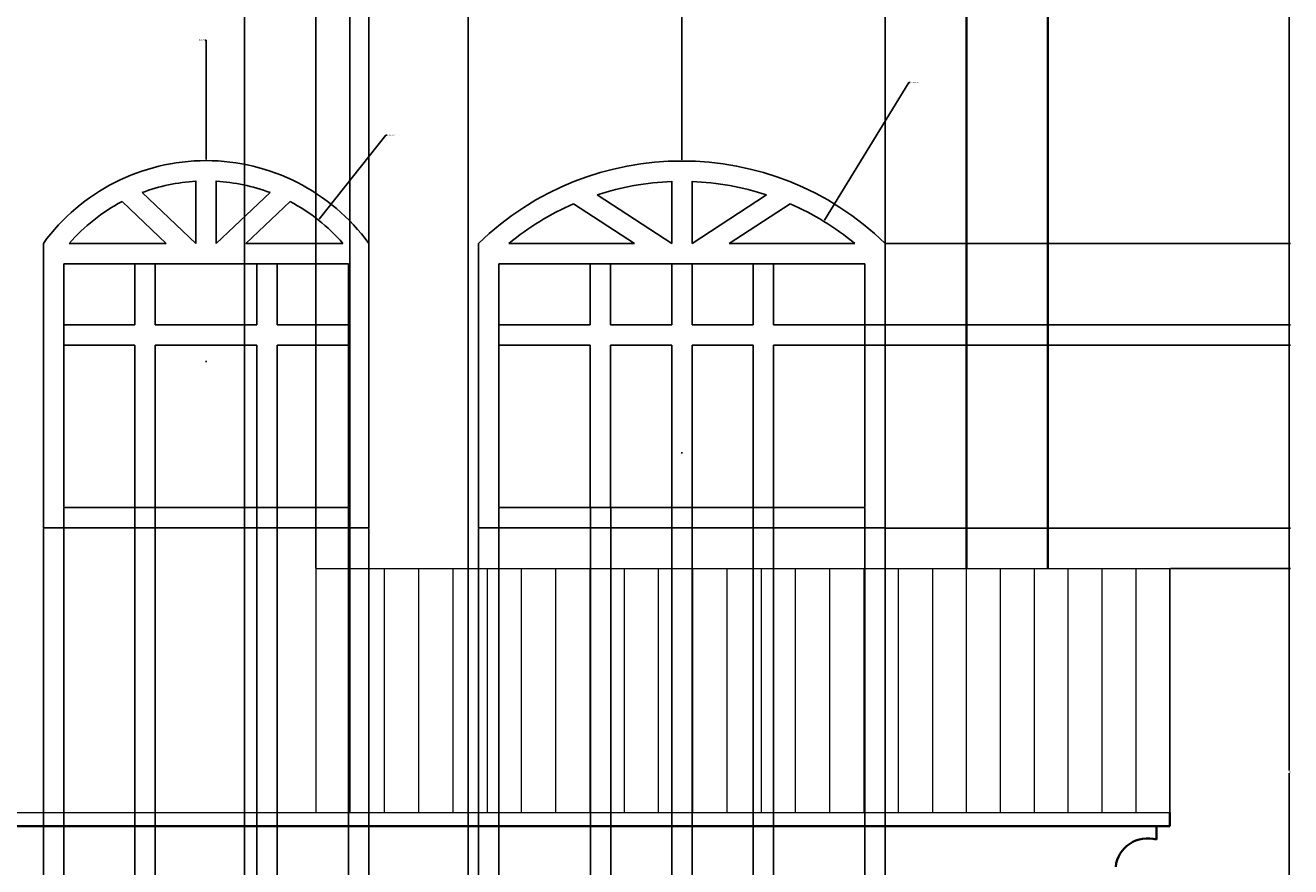
# Model space of a CAD drawing. Units: inches. Extents: x 2612 to 2948, y 481 to 865.
# Tile 6 of 7: x 2761 to 2948, y 659 to 783. Entities that reach past the tile are written whole.
import ezdxf

# ---------------------------------------------------------------- set-up
doc = ezdxf.new("R2010")
doc.units = ezdxf.units.IN
for name, color, linetype, lineweight in [('A-ANNO-DIMS', 2, 'Continuous', 18), ('A-COLS', 1, 'Continuous', 35), ('A-ELEV', 7, 'Continuous', 35), ('A-ELEV-RAIL', 3, 'Continuous', 18), ('A-GLAZ', 4, 'Continuous', 25)]:
    doc.layers.add(name, color=color, linetype=linetype, lineweight=lineweight)
doc.styles.get("Standard").update_dxf_attribs({"font": 'arial.ttf'})
doc.dimstyles.get("Standard").update_dxf_attribs({"dimtxt": 0.18, "dimasz": 0.18, "dimexe": 0.18, "dimexo": 0.0625, "dimgap": 0.09, "dimtad": 0, "dimtih": 1, "dimtoh": 1, "dimdec": 4, "dimzin": 0, "dimdsep": 46, "dimtxsty": 'Standard', "dimcen": 0.09, "dimadec": 0, "dimazin": 0, "dimtfac": 1, "dimtdec": 4, "dimtofl": 0, "dimtmove": 0, "dimatfit": 3, "dimfxl": 1, "dimtolj": 1, "dimtzin": 0, "dimarcsym": 0})

# ---------------------------------------------------------------- blocks, each defined once
blk = doc.blocks.new('*D15')
at = {"layer": 'A-ANNO-DIMS', "color": 0, "lineweight": -2, "transparency": 16777216}
for p, q in [((2888.37, 709.04), (2948.09, 709.04)), ((2947.91, 708.86), (2947.91, 706.23)), ((2947.91, 703.22), (2947.91, 705.86)), ((2930.37, 703.04), (2948.09, 703.04))]:
    blk.add_line(p, q, dxfattribs=at)
at = {"layer": 'A-ANNO-DIMS', "color": 0, "transparency": 16777216}
for points in [[(2947.88, 708.86), (2947.94, 708.86), (2947.91, 709.04)], [(2947.88, 703.22), (2947.94, 703.22), (2947.91, 703.04)]]:
    blk.add_solid(points, dxfattribs=at)
at = {"layer": 'Defpoints', "color": 0, "transparency": 16777216}
for p in [(2888.31, 709.04), (2947.91, 709.04), (2930.31, 703.04)]:
    blk.add_point(p, dxfattribs=at)
at = {"layer": 'A-ANNO-DIMS', "color": 0, "transparency": 16777216, "insert": (2947.91, 706.04), "char_height": 0.18, "attachment_point": 5}
blk.add_mtext('\\A1;6', dxfattribs=at)
blk = doc.blocks.new('*D33')
at = {"layer": 'A-ANNO-DIMS', "color": 0, "lineweight": -2, "transparency": 16777216}
for p, q in [((2756.31, 703.11), (2756.31, 864.82)), ((2756.49, 864.64), (2780.08, 864.64)), ((2804.13, 864.64), (2780.53, 864.64)), ((2804.31, 703.11), (2804.31, 864.82))]:
    blk.add_line(p, q, dxfattribs=at)
at = {"layer": 'A-ANNO-DIMS', "color": 0, "transparency": 16777216}
for points in [[(2756.49, 864.67), (2756.49, 864.61), (2756.31, 864.64)], [(2804.13, 864.67), (2804.13, 864.61), (2804.31, 864.64)]]:
    blk.add_solid(points, dxfattribs=at)
at = {"layer": 'Defpoints', "color": 0, "transparency": 16777216}
for p in [(2804.31, 864.64), (2756.31, 703.04), (2804.31, 703.04)]:
    blk.add_point(p, dxfattribs=at)
at = {"layer": 'A-ANNO-DIMS', "color": 0, "transparency": 16777216, "insert": (2780.31, 864.64), "char_height": 0.18, "attachment_point": 5}
blk.add_mtext('\\A1;48', dxfattribs=at)
blk = doc.blocks.new('*D34')
at = {"layer": 'A-ANNO-DIMS', "color": 0, "lineweight": -2, "transparency": 16777216}
for p, q in [((2804.31, 703.11), (2804.31, 864.82)), ((2804.49, 864.64), (2806.44, 864.64)), ((2809.18, 864.64), (2807.23, 864.64)), ((2809.36, 703.11), (2809.36, 864.82))]:
    blk.add_line(p, q, dxfattribs=at)
at = {"layer": 'A-ANNO-DIMS', "color": 0, "transparency": 16777216}
for points in [[(2804.49, 864.67), (2804.49, 864.61), (2804.31, 864.64)], [(2809.18, 864.67), (2809.18, 864.61), (2809.36, 864.64)]]:
    blk.add_solid(points, dxfattribs=at)
at = {"layer": 'Defpoints', "color": 0, "transparency": 16777216}
for p in [(2809.36, 864.64), (2804.31, 703.04), (2809.36, 703.04)]:
    blk.add_point(p, dxfattribs=at)
at = {"layer": 'A-ANNO-DIMS', "color": 0, "transparency": 16777216, "insert": (2806.83, 864.64), "char_height": 0.18, "attachment_point": 5}
blk.add_mtext('\\A1;5.053', dxfattribs=at)
blk = doc.blocks.new('*D35')
at = {"layer": 'A-ANNO-DIMS', "color": 0, "lineweight": -2, "transparency": 16777216}
for p, q in [((2809.36, 703.11), (2809.36, 864.82)), ((2809.54, 864.64), (2810.42, 864.64)), ((2811.95, 864.64), (2811.07, 864.64)), ((2812.13, 709.11), (2812.13, 864.82))]:
    blk.add_line(p, q, dxfattribs=at)
at = {"layer": 'A-ANNO-DIMS', "color": 0, "transparency": 16777216}
for points in [[(2809.54, 864.67), (2809.54, 864.61), (2809.36, 864.64)], [(2811.95, 864.67), (2811.95, 864.61), (2812.13, 864.64)]]:
    blk.add_solid(points, dxfattribs=at)
at = {"layer": 'Defpoints', "color": 0, "transparency": 16777216}
for p in [(2812.13, 864.64), (2812.13, 709.04), (2809.36, 703.04)]:
    blk.add_point(p, dxfattribs=at)
at = {"layer": 'A-ANNO-DIMS', "color": 0, "transparency": 16777216, "insert": (2810.75, 864.64), "char_height": 0.18, "attachment_point": 5}
blk.add_mtext('\\A1;2.77', dxfattribs=at)
blk = doc.blocks.new('*D36')
at = {"layer": 'A-ANNO-DIMS', "color": 0, "lineweight": -2, "transparency": 16777216}
for p, q in [((2888.31, 709.11), (2888.31, 864.82)), ((2888.49, 864.64), (2894.1, 864.64)), ((2900.13, 864.64), (2894.52, 864.64)), ((2900.31, 787.11), (2900.31, 864.82))]:
    blk.add_line(p, q, dxfattribs=at)
at = {"layer": 'A-ANNO-DIMS', "color": 0, "transparency": 16777216}
for points in [[(2888.49, 864.67), (2888.49, 864.61), (2888.31, 864.64)], [(2900.13, 864.67), (2900.13, 864.61), (2900.31, 864.64)]]:
    blk.add_solid(points, dxfattribs=at)
at = {"layer": 'Defpoints', "color": 0, "transparency": 16777216}
for p in [(2900.31, 864.64), (2900.31, 787.04), (2888.31, 709.04)]:
    blk.add_point(p, dxfattribs=at)
at = {"layer": 'A-ANNO-DIMS', "color": 0, "transparency": 16777216, "insert": (2894.31, 864.64), "char_height": 0.18, "attachment_point": 5}
blk.add_mtext('\\A1;12', dxfattribs=at)
blk = doc.blocks.new('*D50')
at = {"layer": 'A-ANNO-DIMS', "color": 0, "lineweight": -2, "transparency": 16777216}
for p, q in [((2745.81, 604.11), (2745.81, 864.82)), ((2745.99, 864.64), (2769.58, 864.64)), ((2793.63, 864.64), (2770.03, 864.64)), ((2793.81, 604.11), (2793.81, 864.82))]:
    blk.add_line(p, q, dxfattribs=at)
at = {"layer": 'A-ANNO-DIMS', "color": 0, "transparency": 16777216}
for points in [[(2745.99, 864.67), (2745.99, 864.61), (2745.81, 864.64)], [(2793.63, 864.67), (2793.63, 864.61), (2793.81, 864.64)]]:
    blk.add_solid(points, dxfattribs=at)
at = {"layer": 'Defpoints', "color": 0, "transparency": 16777216}
for p in [(2793.81, 864.64), (2745.81, 604.04), (2793.81, 604.04)]:
    blk.add_point(p, dxfattribs=at)
at = {"layer": 'A-ANNO-DIMS', "color": 0, "transparency": 16777216, "insert": (2769.81, 864.64), "char_height": 0.18, "attachment_point": 5}
blk.add_mtext('\\A1;48', dxfattribs=at)
blk = doc.blocks.new('*D51')
at = {"layer": 'A-ANNO-DIMS', "color": 0, "lineweight": -2, "transparency": 16777216}
for p, q in [((2793.81, 604.11), (2793.81, 864.82)), ((2793.99, 864.64), (2810.09, 864.64)), ((2826.63, 864.64), (2810.53, 864.64)), ((2826.81, 562.11), (2826.81, 864.82))]:
    blk.add_line(p, q, dxfattribs=at)
at = {"layer": 'A-ANNO-DIMS', "color": 0, "transparency": 16777216}
for points in [[(2793.99, 864.67), (2793.99, 864.61), (2793.81, 864.64)], [(2826.63, 864.67), (2826.63, 864.61), (2826.81, 864.64)]]:
    blk.add_solid(points, dxfattribs=at)
at = {"layer": 'Defpoints', "color": 0, "transparency": 16777216}
for p in [(2826.81, 864.64), (2793.81, 604.04), (2826.81, 562.04)]:
    blk.add_point(p, dxfattribs=at)
at = {"layer": 'A-ANNO-DIMS', "color": 0, "transparency": 16777216, "insert": (2810.31, 864.64), "char_height": 0.18, "attachment_point": 5}
blk.add_mtext('\\A1;33', dxfattribs=at)
blk = doc.blocks.new('*D66')
at = {"layer": 'A-ANNO-DIMS', "color": 0, "lineweight": -2, "transparency": 16777216}
for p, q in [((2767.13, 711.98), (2767.13, 481.26)), ((2764.13, 708.98), (2764.13, 481.26)), ((2764.31, 481.44), (2765.48, 481.44)), ((2766.95, 481.44), (2765.78, 481.44))]:
    blk.add_line(p, q, dxfattribs=at)
at = {"layer": 'A-ANNO-DIMS', "color": 0, "transparency": 16777216}
for points in [[(2764.31, 481.47), (2764.31, 481.41), (2764.13, 481.44)], [(2766.95, 481.47), (2766.95, 481.41), (2767.13, 481.44)]]:
    blk.add_solid(points, dxfattribs=at)
at = {"layer": 'Defpoints', "color": 0, "transparency": 16777216}
for p in [(2767.13, 712.04), (2764.13, 709.04), (2767.13, 481.44)]:
    blk.add_point(p, dxfattribs=at)
at = {"layer": 'A-ANNO-DIMS', "color": 0, "transparency": 16777216, "insert": (2765.63, 481.44), "char_height": 0.18, "attachment_point": 5}
blk.add_mtext('\\A1;3', dxfattribs=at)
blk = doc.blocks.new('*D67')
at = {"layer": 'A-ANNO-DIMS', "color": 0, "lineweight": -2, "transparency": 16777216}
for p, q in [((2767.13, 711.98), (2767.13, 481.26)), ((2777.63, 711.98), (2777.63, 481.26)), ((2767.31, 481.44), (2772.06, 481.44)), ((2777.45, 481.44), (2772.7, 481.44))]:
    blk.add_line(p, q, dxfattribs=at)
at = {"layer": 'A-ANNO-DIMS', "color": 0, "transparency": 16777216}
for points in [[(2767.31, 481.47), (2767.31, 481.41), (2767.13, 481.44)], [(2777.45, 481.47), (2777.45, 481.41), (2777.63, 481.44)]]:
    blk.add_solid(points, dxfattribs=at)
at = {"layer": 'Defpoints', "color": 0, "transparency": 16777216}
for p in [(2767.13, 712.04), (2777.63, 712.04), (2777.63, 481.44)]:
    blk.add_point(p, dxfattribs=at)
at = {"layer": 'A-ANNO-DIMS', "color": 0, "transparency": 16777216, "insert": (2772.38, 481.44), "char_height": 0.18, "attachment_point": 5}
blk.add_mtext('\\A1;10.5', dxfattribs=at)
blk = doc.blocks.new('*D68')
at = {"layer": 'A-ANNO-DIMS', "color": 0, "lineweight": -2, "transparency": 16777216}
for p, q in [((2777.63, 711.98), (2777.63, 481.26)), ((2780.63, 711.98), (2780.63, 481.26)), ((2777.81, 481.44), (2778.98, 481.44)), ((2780.45, 481.44), (2779.28, 481.44))]:
    blk.add_line(p, q, dxfattribs=at)
at = {"layer": 'A-ANNO-DIMS', "color": 0, "transparency": 16777216}
for points in [[(2777.81, 481.47), (2777.81, 481.41), (2777.63, 481.44)], [(2780.45, 481.47), (2780.45, 481.41), (2780.63, 481.44)]]:
    blk.add_solid(points, dxfattribs=at)
at = {"layer": 'Defpoints', "color": 0, "transparency": 16777216}
for p in [(2777.63, 712.04), (2780.63, 712.04), (2780.63, 481.44)]:
    blk.add_point(p, dxfattribs=at)
at = {"layer": 'A-ANNO-DIMS', "color": 0, "transparency": 16777216, "insert": (2779.13, 481.44), "char_height": 0.18, "attachment_point": 5}
blk.add_mtext('\\A1;3', dxfattribs=at)
blk = doc.blocks.new('*D69')
at = {"layer": 'A-ANNO-DIMS', "color": 0, "lineweight": -2, "transparency": 16777216}
for p, q in [((2780.63, 711.98), (2780.63, 481.26)), ((2795.63, 711.98), (2795.63, 481.26)), ((2780.81, 481.44), (2787.92, 481.44)), ((2795.45, 481.44), (2788.34, 481.44))]:
    blk.add_line(p, q, dxfattribs=at)
at = {"layer": 'A-ANNO-DIMS', "color": 0, "transparency": 16777216}
for points in [[(2780.81, 481.47), (2780.81, 481.41), (2780.63, 481.44)], [(2795.45, 481.47), (2795.45, 481.41), (2795.63, 481.44)]]:
    blk.add_solid(points, dxfattribs=at)
at = {"layer": 'Defpoints', "color": 0, "transparency": 16777216}
for p in [(2780.63, 712.04), (2795.63, 712.04), (2795.63, 481.44)]:
    blk.add_point(p, dxfattribs=at)
at = {"layer": 'A-ANNO-DIMS', "color": 0, "transparency": 16777216, "insert": (2788.13, 481.44), "char_height": 0.18, "attachment_point": 5}
blk.add_mtext('\\A1;15', dxfattribs=at)
blk = doc.blocks.new('*D70')
at = {"layer": 'A-ANNO-DIMS', "color": 0, "lineweight": -2, "transparency": 16777216}
for p, q in [((2795.63, 711.98), (2795.63, 481.26)), ((2798.63, 711.98), (2798.63, 481.26)), ((2795.81, 481.44), (2796.98, 481.44)), ((2798.45, 481.44), (2797.28, 481.44))]:
    blk.add_line(p, q, dxfattribs=at)
at = {"layer": 'A-ANNO-DIMS', "color": 0, "transparency": 16777216}
for points in [[(2795.81, 481.47), (2795.81, 481.41), (2795.63, 481.44)], [(2798.45, 481.47), (2798.45, 481.41), (2798.63, 481.44)]]:
    blk.add_solid(points, dxfattribs=at)
at = {"layer": 'Defpoints', "color": 0, "transparency": 16777216}
for p in [(2795.63, 712.04), (2798.63, 712.04), (2798.63, 481.44)]:
    blk.add_point(p, dxfattribs=at)
at = {"layer": 'A-ANNO-DIMS', "color": 0, "transparency": 16777216, "insert": (2797.13, 481.44), "char_height": 0.18, "attachment_point": 5}
blk.add_mtext('\\A1;3', dxfattribs=at)
blk = doc.blocks.new('*D71')
at = {"layer": 'A-ANNO-DIMS', "color": 0, "lineweight": -2, "transparency": 16777216}
for p, q in [((2798.63, 711.98), (2798.63, 481.26)), ((2809.13, 711.98), (2809.13, 481.26)), ((2798.81, 481.44), (2803.56, 481.44)), ((2808.95, 481.44), (2804.2, 481.44))]:
    blk.add_line(p, q, dxfattribs=at)
at = {"layer": 'A-ANNO-DIMS', "color": 0, "transparency": 16777216}
for points in [[(2798.81, 481.47), (2798.81, 481.41), (2798.63, 481.44)], [(2808.95, 481.47), (2808.95, 481.41), (2809.13, 481.44)]]:
    blk.add_solid(points, dxfattribs=at)
at = {"layer": 'Defpoints', "color": 0, "transparency": 16777216}
for p in [(2798.63, 712.04), (2809.13, 712.04), (2809.13, 481.44)]:
    blk.add_point(p, dxfattribs=at)
at = {"layer": 'A-ANNO-DIMS', "color": 0, "transparency": 16777216, "insert": (2803.88, 481.44), "char_height": 0.18, "attachment_point": 5}
blk.add_mtext('\\A1;10.5', dxfattribs=at)
blk = doc.blocks.new('*D72')
at = {"layer": 'A-ANNO-DIMS', "color": 0, "lineweight": -2, "transparency": 16777216}
for p, q in [((2809.13, 711.98), (2809.13, 481.26)), ((2812.13, 708.98), (2812.13, 481.26)), ((2809.31, 481.44), (2810.48, 481.44)), ((2811.95, 481.44), (2810.78, 481.44))]:
    blk.add_line(p, q, dxfattribs=at)
at = {"layer": 'A-ANNO-DIMS', "color": 0, "transparency": 16777216}
for points in [[(2809.31, 481.47), (2809.31, 481.41), (2809.13, 481.44)], [(2811.95, 481.47), (2811.95, 481.41), (2812.13, 481.44)]]:
    blk.add_solid(points, dxfattribs=at)
at = {"layer": 'Defpoints', "color": 0, "transparency": 16777216}
for p in [(2809.13, 712.04), (2812.13, 709.04), (2812.13, 481.44)]:
    blk.add_point(p, dxfattribs=at)
at = {"layer": 'A-ANNO-DIMS', "color": 0, "transparency": 16777216, "insert": (2810.63, 481.44), "char_height": 0.18, "attachment_point": 5}
blk.add_mtext('\\A1;3', dxfattribs=at)
blk = doc.blocks.new('*D73')
at = {"layer": 'A-ANNO-DIMS', "color": 0, "lineweight": -2, "transparency": 16777216}
for p, q in [((2812.13, 708.98), (2812.13, 481.26)), ((2828.31, 708.98), (2828.31, 481.26)), ((2812.31, 481.44), (2819.76, 481.44)), ((2828.13, 481.44), (2820.67, 481.44))]:
    blk.add_line(p, q, dxfattribs=at)
at = {"layer": 'A-ANNO-DIMS', "color": 0, "transparency": 16777216}
for points in [[(2812.31, 481.47), (2812.31, 481.41), (2812.13, 481.44)], [(2828.13, 481.47), (2828.13, 481.41), (2828.31, 481.44)]]:
    blk.add_solid(points, dxfattribs=at)
at = {"layer": 'Defpoints', "color": 0, "transparency": 16777216}
for p in [(2812.13, 709.04), (2828.31, 709.04), (2828.31, 481.44)]:
    blk.add_point(p, dxfattribs=at)
at = {"layer": 'A-ANNO-DIMS', "color": 0, "transparency": 16777216, "insert": (2820.22, 481.44), "char_height": 0.18, "attachment_point": 5}
blk.add_mtext('\\A1;16.177', dxfattribs=at)
blk = doc.blocks.new('*D74')
at = {"layer": 'A-ANNO-DIMS', "color": 0, "lineweight": -2, "transparency": 16777216}
for p, q in [((2831.31, 711.98), (2831.31, 481.26)), ((2828.31, 708.98), (2828.31, 481.26)), ((2828.49, 481.44), (2829.66, 481.44)), ((2831.13, 481.44), (2829.96, 481.44))]:
    blk.add_line(p, q, dxfattribs=at)
at = {"layer": 'A-ANNO-DIMS', "color": 0, "transparency": 16777216}
for points in [[(2828.49, 481.47), (2828.49, 481.41), (2828.31, 481.44)], [(2831.13, 481.47), (2831.13, 481.41), (2831.31, 481.44)]]:
    blk.add_solid(points, dxfattribs=at)
at = {"layer": 'Defpoints', "color": 0, "transparency": 16777216}
for p in [(2831.31, 712.04), (2828.31, 709.04), (2831.31, 481.44)]:
    blk.add_point(p, dxfattribs=at)
at = {"layer": 'A-ANNO-DIMS', "color": 0, "transparency": 16777216, "insert": (2829.81, 481.44), "char_height": 0.18, "attachment_point": 5}
blk.add_mtext('\\A1;3', dxfattribs=at)
blk = doc.blocks.new('*D75')
at = {"layer": 'A-ANNO-DIMS', "color": 0, "lineweight": -2, "transparency": 16777216}
for p, q in [((2831.31, 711.98), (2831.31, 481.26)), ((2844.81, 711.98), (2844.81, 481.26)), ((2831.49, 481.44), (2837.74, 481.44)), ((2844.63, 481.44), (2838.37, 481.44))]:
    blk.add_line(p, q, dxfattribs=at)
at = {"layer": 'A-ANNO-DIMS', "color": 0, "transparency": 16777216}
for points in [[(2831.49, 481.47), (2831.49, 481.41), (2831.31, 481.44)], [(2844.63, 481.47), (2844.63, 481.41), (2844.81, 481.44)]]:
    blk.add_solid(points, dxfattribs=at)
at = {"layer": 'Defpoints', "color": 0, "transparency": 16777216}
for p in [(2831.31, 712.04), (2844.81, 712.04), (2844.81, 481.44)]:
    blk.add_point(p, dxfattribs=at)
at = {"layer": 'A-ANNO-DIMS', "color": 0, "transparency": 16777216, "insert": (2838.06, 481.44), "char_height": 0.18, "attachment_point": 5}
blk.add_mtext('\\A1;13.5', dxfattribs=at)
blk = doc.blocks.new('*D76')
at = {"layer": 'A-ANNO-DIMS', "color": 0, "lineweight": -2, "transparency": 16777216}
for p, q in [((2844.81, 711.98), (2844.81, 481.26)), ((2847.81, 711.98), (2847.81, 481.26)), ((2844.99, 481.44), (2846.16, 481.44)), ((2847.63, 481.44), (2846.46, 481.44))]:
    blk.add_line(p, q, dxfattribs=at)
at = {"layer": 'A-ANNO-DIMS', "color": 0, "transparency": 16777216}
for points in [[(2844.99, 481.47), (2844.99, 481.41), (2844.81, 481.44)], [(2847.63, 481.47), (2847.63, 481.41), (2847.81, 481.44)]]:
    blk.add_solid(points, dxfattribs=at)
at = {"layer": 'Defpoints', "color": 0, "transparency": 16777216}
for p in [(2844.81, 712.04), (2847.81, 712.04), (2847.81, 481.44)]:
    blk.add_point(p, dxfattribs=at)
at = {"layer": 'A-ANNO-DIMS', "color": 0, "transparency": 16777216, "insert": (2846.31, 481.44), "char_height": 0.18, "attachment_point": 5}
blk.add_mtext('\\A1;3', dxfattribs=at)
blk = doc.blocks.new('*D77')
at = {"layer": 'A-ANNO-DIMS', "color": 0, "lineweight": -2, "transparency": 16777216}
for p, q in [((2847.81, 711.98), (2847.81, 481.26)), ((2856.81, 711.98), (2856.81, 481.26)), ((2847.99, 481.44), (2852.16, 481.44)), ((2856.63, 481.44), (2852.46, 481.44))]:
    blk.add_line(p, q, dxfattribs=at)
at = {"layer": 'A-ANNO-DIMS', "color": 0, "transparency": 16777216}
for points in [[(2847.99, 481.47), (2847.99, 481.41), (2847.81, 481.44)], [(2856.63, 481.47), (2856.63, 481.41), (2856.81, 481.44)]]:
    blk.add_solid(points, dxfattribs=at)
at = {"layer": 'Defpoints', "color": 0, "transparency": 16777216}
for p in [(2847.81, 712.04), (2856.81, 712.04), (2856.81, 481.44)]:
    blk.add_point(p, dxfattribs=at)
at = {"layer": 'A-ANNO-DIMS', "color": 0, "transparency": 16777216, "insert": (2852.31, 481.44), "char_height": 0.18, "attachment_point": 5}
blk.add_mtext('\\A1;9', dxfattribs=at)
blk = doc.blocks.new('*D78')
at = {"layer": 'A-ANNO-DIMS', "color": 0, "lineweight": -2, "transparency": 16777216}
for p, q in [((2856.81, 711.98), (2856.81, 481.26)), ((2859.81, 711.98), (2859.81, 481.26)), ((2856.99, 481.44), (2858.16, 481.44)), ((2859.63, 481.44), (2858.46, 481.44))]:
    blk.add_line(p, q, dxfattribs=at)
at = {"layer": 'A-ANNO-DIMS', "color": 0, "transparency": 16777216}
for points in [[(2856.99, 481.47), (2856.99, 481.41), (2856.81, 481.44)], [(2859.63, 481.47), (2859.63, 481.41), (2859.81, 481.44)]]:
    blk.add_solid(points, dxfattribs=at)
at = {"layer": 'Defpoints', "color": 0, "transparency": 16777216}
for p in [(2856.81, 712.04), (2859.81, 712.04), (2859.81, 481.44)]:
    blk.add_point(p, dxfattribs=at)
at = {"layer": 'A-ANNO-DIMS', "color": 0, "transparency": 16777216, "insert": (2858.31, 481.44), "char_height": 0.18, "attachment_point": 5}
blk.add_mtext('\\A1;3', dxfattribs=at)
blk = doc.blocks.new('*D79')
at = {"layer": 'A-ANNO-DIMS', "color": 0, "lineweight": -2, "transparency": 16777216}
for p, q in [((2859.81, 711.98), (2859.81, 481.26)), ((2868.81, 711.98), (2868.81, 481.26)), ((2859.99, 481.44), (2864.16, 481.44)), ((2868.63, 481.44), (2864.46, 481.44))]:
    blk.add_line(p, q, dxfattribs=at)
at = {"layer": 'A-ANNO-DIMS', "color": 0, "transparency": 16777216}
for points in [[(2859.99, 481.47), (2859.99, 481.41), (2859.81, 481.44)], [(2868.63, 481.47), (2868.63, 481.41), (2868.81, 481.44)]]:
    blk.add_solid(points, dxfattribs=at)
at = {"layer": 'Defpoints', "color": 0, "transparency": 16777216}
for p in [(2859.81, 712.04), (2868.81, 712.04), (2868.81, 481.44)]:
    blk.add_point(p, dxfattribs=at)
at = {"layer": 'A-ANNO-DIMS', "color": 0, "transparency": 16777216, "insert": (2864.31, 481.44), "char_height": 0.18, "attachment_point": 5}
blk.add_mtext('\\A1;9', dxfattribs=at)
blk = doc.blocks.new('*D80')
at = {"layer": 'A-ANNO-DIMS', "color": 0, "lineweight": -2, "transparency": 16777216}
for p, q in [((2868.81, 711.98), (2868.81, 481.26)), ((2871.81, 711.98), (2871.81, 481.26)), ((2868.99, 481.44), (2870.16, 481.44)), ((2871.63, 481.44), (2870.46, 481.44))]:
    blk.add_line(p, q, dxfattribs=at)
at = {"layer": 'A-ANNO-DIMS', "color": 0, "transparency": 16777216}
for points in [[(2868.99, 481.47), (2868.99, 481.41), (2868.81, 481.44)], [(2871.63, 481.47), (2871.63, 481.41), (2871.81, 481.44)]]:
    blk.add_solid(points, dxfattribs=at)
at = {"layer": 'Defpoints', "color": 0, "transparency": 16777216}
for p in [(2868.81, 712.04), (2871.81, 712.04), (2871.81, 481.44)]:
    blk.add_point(p, dxfattribs=at)
at = {"layer": 'A-ANNO-DIMS', "color": 0, "transparency": 16777216, "insert": (2870.31, 481.44), "char_height": 0.18, "attachment_point": 5}
blk.add_mtext('\\A1;3', dxfattribs=at)
blk = doc.blocks.new('*D81')
at = {"layer": 'A-ANNO-DIMS', "color": 0, "lineweight": -2, "transparency": 16777216}
for p, q in [((2871.81, 711.98), (2871.81, 481.26)), ((2885.31, 711.98), (2885.31, 481.26)), ((2871.99, 481.44), (2878.24, 481.44)), ((2885.13, 481.44), (2878.87, 481.44))]:
    blk.add_line(p, q, dxfattribs=at)
at = {"layer": 'A-ANNO-DIMS', "color": 0, "transparency": 16777216}
for points in [[(2871.99, 481.47), (2871.99, 481.41), (2871.81, 481.44)], [(2885.13, 481.47), (2885.13, 481.41), (2885.31, 481.44)]]:
    blk.add_solid(points, dxfattribs=at)
at = {"layer": 'Defpoints', "color": 0, "transparency": 16777216}
for p in [(2871.81, 712.04), (2885.31, 712.04), (2885.31, 481.44)]:
    blk.add_point(p, dxfattribs=at)
at = {"layer": 'A-ANNO-DIMS', "color": 0, "transparency": 16777216, "insert": (2878.56, 481.44), "char_height": 0.18, "attachment_point": 5}
blk.add_mtext('\\A1;13.5', dxfattribs=at)
blk = doc.blocks.new('*D82')
at = {"layer": 'A-ANNO-DIMS', "color": 0, "lineweight": -2, "transparency": 16777216}
for p, q in [((2885.31, 711.98), (2885.31, 481.26)), ((2888.31, 708.98), (2888.31, 481.26)), ((2885.49, 481.44), (2886.66, 481.44)), ((2888.13, 481.44), (2886.96, 481.44))]:
    blk.add_line(p, q, dxfattribs=at)
at = {"layer": 'A-ANNO-DIMS', "color": 0, "transparency": 16777216}
for points in [[(2885.49, 481.47), (2885.49, 481.41), (2885.31, 481.44)], [(2888.13, 481.47), (2888.13, 481.41), (2888.31, 481.44)]]:
    blk.add_solid(points, dxfattribs=at)
at = {"layer": 'Defpoints', "color": 0, "transparency": 16777216}
for p in [(2885.31, 712.04), (2888.31, 709.04), (2888.31, 481.44)]:
    blk.add_point(p, dxfattribs=at)
at = {"layer": 'A-ANNO-DIMS', "color": 0, "transparency": 16777216, "insert": (2886.81, 481.44), "char_height": 0.18, "attachment_point": 5}
blk.add_mtext('\\A1;3', dxfattribs=at)
blk = doc.blocks.new('*D83')
at = {"layer": 'A-ANNO-DIMS', "color": 0, "lineweight": -2, "transparency": 16777216}
for p, q in [((2885.37, 736.04), (2948.09, 736.04)), ((2947.91, 735.86), (2947.91, 722.72)), ((2947.91, 709.22), (2947.91, 722.36)), ((2888.37, 709.04), (2948.09, 709.04))]:
    blk.add_line(p, q, dxfattribs=at)
at = {"layer": 'A-ANNO-DIMS', "color": 0, "transparency": 16777216}
for points in [[(2947.88, 735.86), (2947.94, 735.86), (2947.91, 736.04)], [(2947.88, 709.22), (2947.94, 709.22), (2947.91, 709.04)]]:
    blk.add_solid(points, dxfattribs=at)
at = {"layer": 'Defpoints', "color": 0, "transparency": 16777216}
for p in [(2885.31, 736.04), (2947.91, 736.04), (2888.31, 709.04)]:
    blk.add_point(p, dxfattribs=at)
at = {"layer": 'A-ANNO-DIMS', "color": 0, "transparency": 16777216, "insert": (2947.91, 722.54), "char_height": 0.18, "attachment_point": 5}
blk.add_mtext('\\A1;27', dxfattribs=at)
blk = doc.blocks.new('*D84')
at = {"layer": 'A-ANNO-DIMS', "color": 0, "lineweight": -2, "transparency": 16777216}
for p, q in [((2885.37, 739.04), (2948.09, 739.04)), ((2947.91, 738.86), (2947.91, 737.73)), ((2947.91, 736.22), (2947.91, 737.36)), ((2885.37, 736.04), (2948.09, 736.04))]:
    blk.add_line(p, q, dxfattribs=at)
at = {"layer": 'A-ANNO-DIMS', "color": 0, "transparency": 16777216}
for points in [[(2947.88, 738.86), (2947.94, 738.86), (2947.91, 739.04)], [(2947.88, 736.22), (2947.94, 736.22), (2947.91, 736.04)]]:
    blk.add_solid(points, dxfattribs=at)
at = {"layer": 'Defpoints', "color": 0, "transparency": 16777216}
for p in [(2885.31, 739.04), (2947.91, 739.04), (2885.31, 736.04)]:
    blk.add_point(p, dxfattribs=at)
at = {"layer": 'A-ANNO-DIMS', "color": 0, "transparency": 16777216, "insert": (2947.91, 737.54), "char_height": 0.18, "attachment_point": 5}
blk.add_mtext('\\A1;3', dxfattribs=at)
blk = doc.blocks.new('*D85')
at = {"layer": 'A-ANNO-DIMS', "color": 0, "lineweight": -2, "transparency": 16777216}
for p, q in [((2888.37, 751.04), (2948.09, 751.04)), ((2947.91, 750.86), (2947.91, 745.22)), ((2947.91, 739.22), (2947.91, 744.86)), ((2885.37, 739.04), (2948.09, 739.04))]:
    blk.add_line(p, q, dxfattribs=at)
at = {"layer": 'A-ANNO-DIMS', "color": 0, "transparency": 16777216}
for points in [[(2947.88, 750.86), (2947.94, 750.86), (2947.91, 751.04)], [(2947.88, 739.22), (2947.94, 739.22), (2947.91, 739.04)]]:
    blk.add_solid(points, dxfattribs=at)
at = {"layer": 'Defpoints', "color": 0, "transparency": 16777216}
for p in [(2888.31, 751.04), (2947.91, 751.04), (2885.31, 739.04)]:
    blk.add_point(p, dxfattribs=at)
at = {"layer": 'A-ANNO-DIMS', "color": 0, "transparency": 16777216, "insert": (2947.91, 745.04), "char_height": 0.18, "attachment_point": 5}
blk.add_mtext('\\A1;12', dxfattribs=at)
blk = doc.blocks.new('*D86')
at = {"layer": 'A-ANNO-DIMS', "color": 0, "lineweight": -2, "transparency": 16777216}
for p, q in [((2930.37, 847.04), (2948.09, 847.04)), ((2947.91, 846.86), (2947.91, 673.23)), ((2947.91, 499.22), (2947.91, 672.86)), ((2930.37, 499.04), (2948.09, 499.04))]:
    blk.add_line(p, q, dxfattribs=at)
at = {"layer": 'A-ANNO-DIMS', "color": 0, "transparency": 16777216}
for points in [[(2947.88, 846.86), (2947.94, 846.86), (2947.91, 847.04)], [(2947.88, 499.22), (2947.94, 499.22), (2947.91, 499.04)]]:
    blk.add_solid(points, dxfattribs=at)
at = {"layer": 'Defpoints', "color": 0, "transparency": 16777216}
for p in [(2930.31, 847.04), (2947.91, 847.04), (2930.31, 499.04)]:
    blk.add_point(p, dxfattribs=at)
at = {"layer": 'A-ANNO-DIMS', "color": 0, "transparency": 16777216, "insert": (2947.91, 673.04), "char_height": 0.18, "attachment_point": 5}
blk.add_mtext('\\A1;348', dxfattribs=at)
blk = doc.blocks.new('*D105')
at = {"layer": 'A-ANNO-DIMS', "color": 0, "lineweight": -2, "transparency": 16777216}
for p, q in [((2858.13, 789.05), (2858.31, 789.05)), ((2858.31, 789.05), (2858.31, 763.39)), ((2858.22, 720.15), (2858.4, 720.15)), ((2858.31, 720.06), (2858.31, 720.24))]:
    blk.add_line(p, q, dxfattribs=at)
at = {"layer": 'A-ANNO-DIMS', "color": 0, "transparency": 16777216}
blk.add_solid([(2858.34, 763.39), (2858.28, 763.39), (2858.31, 763.21)], dxfattribs=at)
at = {"layer": 'Defpoints', "color": 0, "transparency": 16777216}
for p in [(2858.31, 763.21), (2858.31, 720.15)]:
    blk.add_point(p, dxfattribs=at)
at = {"layer": 'A-ANNO-DIMS', "color": 0, "transparency": 16777216, "insert": (2857.65, 789.05), "char_height": 0.18, "attachment_point": 5}
blk.add_mtext('\\A1;R43.06', dxfattribs=at)
blk = doc.blocks.new('*D106')
at = {"layer": 'A-ANNO-DIMS', "color": 0, "lineweight": -2, "transparency": 16777216}
for p, q in [((2891.81, 774.8), (2879.34, 754.46)), ((2891.99, 774.8), (2891.81, 774.8)), ((2858.22, 720.15), (2858.4, 720.15)), ((2858.31, 720.06), (2858.31, 720.24))]:
    blk.add_line(p, q, dxfattribs=at)
at = {"layer": 'A-ANNO-DIMS', "color": 0, "transparency": 16777216}
blk.add_solid([(2879.31, 754.48), (2879.37, 754.44), (2879.25, 754.31)], dxfattribs=at)
at = {"layer": 'Defpoints', "color": 0, "transparency": 16777216}
for p in [(2879.25, 754.31), (2858.31, 720.15)]:
    blk.add_point(p, dxfattribs=at)
at = {"layer": 'A-ANNO-DIMS', "color": 0, "transparency": 16777216, "insert": (2892.67, 774.8), "char_height": 0.18, "attachment_point": 5}
blk.add_mtext('\\A1;4X R40.06', dxfattribs=at)
blk = doc.blocks.new('*D107')
at = {"layer": 'A-ANNO-DIMS', "color": 0, "lineweight": -2, "transparency": 16777216}
for p, q in [((2787.95, 781.07), (2788.13, 781.07)), ((2788.13, 781.07), (2788.13, 763.45)), ((2788.04, 733.6), (2788.22, 733.6)), ((2788.13, 733.51), (2788.13, 733.69))]:
    blk.add_line(p, q, dxfattribs=at)
at = {"layer": 'A-ANNO-DIMS', "color": 0, "transparency": 16777216}
blk.add_solid([(2788.16, 763.45), (2788.1, 763.45), (2788.13, 763.27)], dxfattribs=at)
at = {"layer": 'Defpoints', "color": 0, "transparency": 16777216}
for p in [(2788.13, 763.27), (2788.13, 733.6)]:
    blk.add_point(p, dxfattribs=at)
at = {"layer": 'A-ANNO-DIMS', "color": 0, "transparency": 16777216, "insert": (2787.47, 781.07), "char_height": 0.18, "attachment_point": 5}
blk.add_mtext('\\A1;R29.67', dxfattribs=at)
blk = doc.blocks.new('*D108')
at = {"layer": 'A-ANNO-DIMS', "color": 0, "lineweight": -2, "transparency": 16777216}
for p, q in [((2814.65, 767.03), (2804.82, 754.64)), ((2814.83, 767.03), (2814.65, 767.03)), ((2788.04, 733.6), (2788.22, 733.6)), ((2788.13, 733.51), (2788.13, 733.69))]:
    blk.add_line(p, q, dxfattribs=at)
at = {"layer": 'A-ANNO-DIMS', "color": 0, "transparency": 16777216}
blk.add_solid([(2804.79, 754.65), (2804.84, 754.62), (2804.7, 754.49)], dxfattribs=at)
at = {"layer": 'Defpoints', "color": 0, "transparency": 16777216}
for p in [(2804.7, 754.49), (2788.13, 733.6)]:
    blk.add_point(p, dxfattribs=at)
at = {"layer": 'A-ANNO-DIMS', "color": 0, "transparency": 16777216, "insert": (2815.51, 767.03), "char_height": 0.18, "attachment_point": 5}
blk.add_mtext('\\A1;4X R26.67', dxfattribs=at)

msp = doc.modelspace()

# ---------------------------------------------------------------- linework, layer by layer
at = {"layer": 'A-COLS'}
msp.add_line((2900.3074, 703.0443), (2900.3074, 787.0443), dxfattribs=at)
at = {"layer": 'A-ELEV'}
for p, q in [((2912.3074, 703.0443), (2912.3074, 787.0443)), ((2930.3074, 665.0443), (2930.3074, 667.0443)), ((2630.3074, 665.0443), (2930.3074, 665.0443)), ((2928.3074, 665.0443), (2923.3074, 665.0443)), ((2930.3074, 665.0443), (2928.3074, 665.0443)), ((2930.3074, 665.0443), (2928.3074, 665.0443)), ((2928.3074, 665.0443), (2928.3074, 663.0443))]:
    msp.add_line(p, q, dxfattribs=at)
msp.add_arc((2926.9909, 658.519), 4.7129, 73.7794, 173.600735, dxfattribs=at)
at = {"layer": 'A-ELEV-RAIL'}
for p, q in [((2804.3074, 703.0443), (2804.3074, 667.0443)), ((2804.3074, 703.0443), (2900.3074, 703.0443)), ((2809.3601, 703.0443), (2809.3601, 667.0443)), ((2814.4127, 703.0443), (2814.4127, 667.0443)), ((2819.4653, 703.0443), (2819.4653, 667.0443)), ((2824.5179, 703.0443), (2824.5179, 667.0443)), ((2829.5706, 703.0443), (2829.5706, 667.0443)), ((2834.6232, 703.0443), (2834.6232, 667.0443)), ((2839.6758, 703.0443), (2839.6758, 667.0443)), ((2844.7285, 703.0443), (2844.7285, 667.0443)), ((2849.7811, 703.0443), (2849.7811, 667.0443)), ((2854.8337, 703.0443), (2854.8337, 667.0443)), ((2859.8864, 703.0443), (2859.8864, 667.0443)), ((2864.939, 703.0443), (2864.939, 667.0443)), ((2869.9916, 703.0443), (2869.9916, 667.0443)), ((2875.0443, 703.0443), (2875.0443, 667.0443)), ((2880.0969, 703.0443), (2880.0969, 667.0443)), ((2885.1495, 703.0443), (2885.1495, 667.0443)), ((2890.2022, 703.0443), (2890.2022, 667.0443)), ((2895.2548, 703.0443), (2895.2548, 667.0443)), ((2900.2548, 703.0443), (2900.2548, 667.0443)), ((2900.3074, 703.0443), (2930.3074, 703.0443)), ((2905.2548, 703.0443), (2905.2548, 667.0443)), ((2910.2548, 703.0443), (2910.2548, 667.0443)), ((2915.2548, 703.0443), (2915.2548, 667.0443)), ((2920.2548, 703.0443), (2920.2548, 667.0443)), ((2925.2548, 703.0443), (2925.2548, 667.0443)), ((2930.2548, 703.0443), (2930.2548, 667.0443)), ((2930.3074, 703.0443), (2930.3074, 667.0443)), ((2630.3074, 667.0443), (2930.3074, 667.0443))]:
    msp.add_line(p, q, dxfattribs=at)
at = {"layer": 'A-GLAZ'}
for p, q in [((2786.6304, 751.0443), (2786.6304, 760.2686)), ((2789.6304, 751.0443), (2789.6304, 760.2686)), ((2856.8074, 751.0443), (2856.8074, 760.2141)), ((2859.8074, 751.0443), (2859.8074, 760.2141)), ((2786.6304, 751.0443), (2778.6966, 758.5445)), ((2789.6304, 751.0443), (2797.5642, 758.5445)), ((2856.8074, 751.0443), (2845.8176, 758.2174)), ((2859.8074, 751.0443), (2870.7973, 758.2174)), ((2782.2634, 751.0443), (2775.7368, 757.2142)), ((2793.9974, 751.0443), (2800.524, 757.2142)), ((2851.3187, 751.0443), (2842.3494, 756.8986)), ((2865.2961, 751.0443), (2874.2654, 756.8986)), ((2764.1304, 709.0443), (2764.1304, 751.0443)), ((2767.9569, 751.0443), (2782.2634, 751.0443)), ((2793.9974, 751.0443), (2808.3039, 751.0443)), ((2812.1304, 709.0443), (2812.1304, 751.0443)), ((2828.3074, 709.0443), (2828.3074, 751.0443)), ((2832.8, 751.0443), (2851.3187, 751.0443)), ((2865.2961, 751.0443), (2883.8149, 751.0443)), ((2888.3074, 709.0443), (2888.3074, 751.0443)), ((2767.1304, 712.0443), (2767.1304, 748.0443)), ((2767.1304, 748.0443), (2809.1304, 748.0443)), ((2777.6304, 748.0443), (2777.6304, 739.0443)), ((2780.6304, 748.0443), (2780.6304, 739.0443)), ((2795.6304, 748.0443), (2795.6304, 739.0443)), ((2798.6304, 748.0443), (2798.6304, 739.0443)), ((2809.1304, 712.0443), (2809.1304, 748.0443)), ((2831.3074, 712.0443), (2831.3074, 748.0443)), ((2831.3074, 748.0443), (2885.3074, 748.0443)), ((2844.8074, 748.0443), (2844.8074, 739.0443)), ((2847.8074, 748.0443), (2847.8074, 739.0443)), ((2856.8074, 748.0443), (2856.8074, 739.0443)), ((2859.8074, 748.0443), (2859.8074, 739.0443)), ((2868.8074, 748.0443), (2868.8074, 739.0443)), ((2871.8074, 748.0443), (2871.8074, 739.0443)), ((2885.3074, 712.0443), (2885.3074, 748.0443)), ((2767.1304, 739.0443), (2777.6304, 739.0443)), ((2780.6304, 739.0443), (2795.6304, 739.0443)), ((2798.6304, 739.0443), (2809.1304, 739.0443)), ((2831.3074, 739.0443), (2844.8074, 739.0443)), ((2847.8074, 739.0443), (2856.8074, 739.0443)), ((2859.8074, 739.0443), (2868.8074, 739.0443)), ((2871.8074, 739.0443), (2885.3074, 739.0443)), ((2767.1304, 736.0443), (2777.6304, 736.0443)), ((2777.6304, 736.0443), (2777.6304, 712.0443)), ((2780.6304, 736.0443), (2795.6304, 736.0443)), ((2780.6304, 736.0443), (2780.6304, 712.0443)), ((2795.6304, 736.0443), (2795.6304, 712.0443)), ((2798.6304, 736.0443), (2809.1304, 736.0443)), ((2798.6304, 736.0443), (2798.6304, 712.0443)), ((2831.3074, 736.0443), (2844.8074, 736.0443)), ((2844.8074, 736.0443), (2844.8074, 712.0443)), ((2847.8074, 736.0443), (2847.8074, 712.0443)), ((2847.8074, 736.0443), (2856.8074, 736.0443)), ((2856.8074, 736.0443), (2856.8074, 712.0443)), ((2859.8074, 736.0443), (2859.8074, 712.0443)), ((2859.8074, 736.0443), (2868.8074, 736.0443)), ((2868.8074, 736.0443), (2868.8074, 712.0443)), ((2871.8074, 736.0443), (2871.8074, 712.0443)), ((2871.8074, 736.0443), (2885.3074, 736.0443)), ((2767.1304, 712.0443), (2809.1304, 712.0443)), ((2831.3074, 712.0443), (2885.3074, 712.0443)), ((2764.1304, 709.0443), (2812.1304, 709.0443)), ((2828.3074, 709.0443), (2888.3074, 709.0443))]:
    msp.add_line(p, q, dxfattribs=at)
for centre, radius, start, end in [((2788.1304, 733.5969), 29.6717, 36.016191, 143.983809), ((2858.3074, 720.1526), 43.0616, 45.838981, 134.161019), ((2788.1304, 733.5969), 26.6717, 93.223977, 110.713802), ((2788.1304, 733.5969), 26.6717, 69.286198, 86.776023), ((2858.3074, 720.1526), 40.0616, 92.145792, 108.165745), ((2858.3074, 720.1526), 40.0616, 71.834255, 87.854208), ((2788.1304, 733.5969), 26.6717, 117.688996, 139.144554), ((2788.1304, 733.5969), 26.6717, 40.855446, 62.311004), ((2858.3074, 720.1526), 40.0616, 113.474282, 129.546694), ((2858.3074, 720.1526), 40.0616, 50.453306, 66.525718)]:
    msp.add_arc(centre, radius, start, end, dxfattribs=at)

# ---------------------------------------------------------------- dimensions: what is measured, and where the dimension line sits
at = {"layer": 'A-ANNO-DIMS'}
for base, p1, p2, override, picture, middle in [((2793.8074, 864.6443), (2745.8074, 604.0443), (2793.8074, 604.0443), {"dimdec": 0, "dimlfac": 1, "dimrnd": 0, "dimzin": 0, "dimdsep": 46, "dimlunit": 2}, '*D50', (2769.8074, 864.6443)), ((2804.3074, 864.6443), (2756.3074, 703.0443), (2804.3074, 703.0443), {"dimdec": 0, "dimlfac": 1, "dimrnd": 0, "dimzin": 0, "dimdsep": 46, "dimlunit": 2}, '*D33', (2780.3074, 864.6443)), ((2826.8074, 864.6443), (2793.8074, 604.0443), (2826.8074, 562.0443), {"dimdec": 0, "dimlfac": 1, "dimrnd": 0, "dimzin": 0, "dimdsep": 46, "dimlunit": 2}, '*D51', (2810.3074, 864.6443)), ((2809.3601, 864.6443), (2804.3074, 703.0443), (2809.3601, 703.0443), {"dimdec": 3, "dimlfac": 1, "dimrnd": 0, "dimzin": 0, "dimdsep": 46, "dimlunit": 2}, '*D34', (2806.8337, 864.6443)), ((2812.1304, 864.6443), (2809.3601, 703.0443), (2812.1304, 709.0443), {"dimdec": 2, "dimlfac": 1, "dimrnd": 0, "dimzin": 0, "dimdsep": 46, "dimlunit": 2}, '*D35', (2810.7452, 864.6443)), ((2900.3074, 864.6443), (2888.3074, 709.0443), (2900.3074, 787.0443), {"dimdec": 0, "dimlfac": 1, "dimrnd": 0, "dimzin": 0, "dimdsep": 46, "dimlunit": 2}, '*D36', (2894.3074, 864.6443)), ((2767.1304, 481.4443), (2764.1304, 709.0443), (2767.1304, 712.0443), {"dimdec": 0, "dimlfac": 1, "dimrnd": 0, "dimzin": 0, "dimdsep": 46, "dimlunit": 2}, '*D66', (2765.6304, 481.4443)), ((2777.6304, 481.4443), (2767.1304, 712.0443), (2777.6304, 712.0443), {"dimdec": 1, "dimlfac": 1, "dimrnd": 0, "dimzin": 0, "dimdsep": 46, "dimlunit": 2}, '*D67', (2772.3804, 481.4443)), ((2780.6304, 481.4443), (2777.6304, 712.0443), (2780.6304, 712.0443), {"dimdec": 0, "dimlfac": 1, "dimrnd": 0, "dimzin": 0, "dimdsep": 46, "dimlunit": 2}, '*D68', (2779.1304, 481.4443)), ((2795.6304, 481.4443), (2780.6304, 712.0443), (2795.6304, 712.0443), {"dimdec": 0, "dimlfac": 1, "dimrnd": 0, "dimzin": 0, "dimdsep": 46, "dimlunit": 2}, '*D69', (2788.1304, 481.4443)), ((2798.6304, 481.4443), (2795.6304, 712.0443), (2798.6304, 712.0443), {"dimdec": 0, "dimlfac": 1, "dimrnd": 0, "dimzin": 0, "dimdsep": 46, "dimlunit": 2}, '*D70', (2797.1304, 481.4443)), ((2809.1304, 481.4443), (2798.6304, 712.0443), (2809.1304, 712.0443), {"dimdec": 1, "dimlfac": 1, "dimrnd": 0, "dimzin": 0, "dimdsep": 46, "dimlunit": 2}, '*D71', (2803.8804, 481.4443)), ((2812.1304, 481.4443), (2809.1304, 712.0443), (2812.1304, 709.0443), {"dimdec": 0, "dimlfac": 1, "dimrnd": 0, "dimzin": 0, "dimdsep": 46, "dimlunit": 2}, '*D72', (2810.6304, 481.4443)), ((2831.3074, 481.4443), (2828.3074, 709.0443), (2831.3074, 712.0443), {"dimdec": 0, "dimlfac": 1, "dimrnd": 0, "dimzin": 0, "dimdsep": 46, "dimlunit": 2}, '*D74', (2829.8074, 481.4443)), ((2844.8074, 481.4443), (2831.3074, 712.0443), (2844.8074, 712.0443), {"dimdec": 1, "dimlfac": 1, "dimrnd": 0, "dimzin": 0, "dimdsep": 46, "dimlunit": 2}, '*D75', (2838.0574, 481.4443)), ((2847.8074, 481.4443), (2844.8074, 712.0443), (2847.8074, 712.0443), {"dimdec": 0, "dimlfac": 1, "dimrnd": 0, "dimzin": 0, "dimdsep": 46, "dimlunit": 2}, '*D76', (2846.3074, 481.4443)), ((2856.8074, 481.4443), (2847.8074, 712.0443), (2856.8074, 712.0443), {"dimdec": 0, "dimlfac": 1, "dimrnd": 0, "dimzin": 0, "dimdsep": 46, "dimlunit": 2}, '*D77', (2852.3074, 481.4443)), ((2859.8074, 481.4443), (2856.8074, 712.0443), (2859.8074, 712.0443), {"dimdec": 0, "dimlfac": 1, "dimrnd": 0, "dimzin": 0, "dimdsep": 46, "dimlunit": 2}, '*D78', (2858.3074, 481.4443)), ((2868.8074, 481.4443), (2859.8074, 712.0443), (2868.8074, 712.0443), {"dimdec": 0, "dimlfac": 1, "dimrnd": 0, "dimzin": 0, "dimdsep": 46, "dimlunit": 2}, '*D79', (2864.3074, 481.4443)), ((2871.8074, 481.4443), (2868.8074, 712.0443), (2871.8074, 712.0443), {"dimdec": 0, "dimlfac": 1, "dimrnd": 0, "dimzin": 0, "dimdsep": 46, "dimlunit": 2}, '*D80', (2870.3074, 481.4443)), ((2885.3074, 481.4443), (2871.8074, 712.0443), (2885.3074, 712.0443), {"dimdec": 1, "dimlfac": 1, "dimrnd": 0, "dimzin": 0, "dimdsep": 46, "dimlunit": 2}, '*D81', (2878.5574, 481.4443)), ((2888.3074, 481.4443), (2885.3074, 712.0443), (2888.3074, 709.0443), {"dimdec": 0, "dimlfac": 1, "dimrnd": 0, "dimzin": 0, "dimdsep": 46, "dimlunit": 2}, '*D82', (2886.8074, 481.4443)), ((2828.3074, 481.4443), (2812.1304, 709.0443), (2828.3074, 709.0443), {"dimdec": 3, "dimlfac": 1, "dimrnd": 0, "dimzin": 0, "dimdsep": 46, "dimlunit": 2}, '*D73', (2820.2189, 481.4443))]:
    dim = msp.add_linear_dim(base=base, p1=p1, p2=p2, dimstyle='Standard', override=override, dxfattribs=at)
    dim.commit()
    dim.dimension.update_dxf_attribs({"geometry": picture, "text_midpoint": middle})
for base, p1, p2, picture, middle in [((2947.9074, 847.0443), (2930.3074, 499.0443), (2930.3074, 847.0443), '*D86', (2947.9074, 673.0443)), ((2947.9074, 751.0443), (2885.3074, 739.0443), (2888.3074, 751.0443), '*D85', (2947.9074, 745.0443)), ((2947.9074, 739.0443), (2885.3074, 736.0443), (2885.3074, 739.0443), '*D84', (2947.9074, 737.5443)), ((2947.9074, 736.0443), (2888.3074, 709.0443), (2885.3074, 736.0443), '*D83', (2947.9074, 722.5443)), ((2947.9074, 709.0443), (2930.3074, 703.0443), (2888.3074, 709.0443), '*D15', (2947.9074, 706.0443))]:
    dim = msp.add_linear_dim(base=base, p1=p1, p2=p2, angle=90, dimstyle='Standard', override={"dimdec": 0, "dimlfac": 1, "dimrnd": 0, "dimzin": 0, "dimdsep": 46, "dimlunit": 2}, dxfattribs=at)
    dim.commit()
    dim.dimension.update_dxf_attribs({"geometry": picture, "text_midpoint": middle})
for center, mpoint, picture, middle in [((2858.3074, 720.1526), (2858.307, 763.2141), '*D105', (2857.647, 789.0511)), ((2788.1304, 733.5969), (2788.13, 763.2686), '*D107', (2787.4699, 781.0716))]:
    dim = msp.add_radius_dim(center=center, mpoint=mpoint, dimstyle='Standard', override={"dimdec": 2, "dimlfac": 1, "dimrnd": 0, "dimzin": 0, "dimdsep": 46, "dimlunit": 2}, dxfattribs=at)
    dim.commit()
    dim.dimension.update_dxf_attribs({"geometry": picture, "text_midpoint": middle, "dimtype": 164})
for center, mpoint, picture, middle in [((2858.3074, 720.1526), (2879.2459, 754.3068), '*D106', (2892.6657, 774.7993)), ((2788.1304, 733.5969), (2804.7041, 754.4941), '*D108', (2815.5051, 767.0324))]:
    dim = msp.add_radius_dim(center=center, mpoint=mpoint, text='4X <>', dimstyle='Standard', override={"dimdec": 2, "dimlfac": 1, "dimrnd": 0, "dimzin": 0, "dimdsep": 46, "dimlunit": 2}, dxfattribs=at)
    dim.commit()
    dim.dimension.update_dxf_attribs({"geometry": picture, "text_midpoint": middle, "dimtype": 164})

doc.saveas('drawing.dxf')
